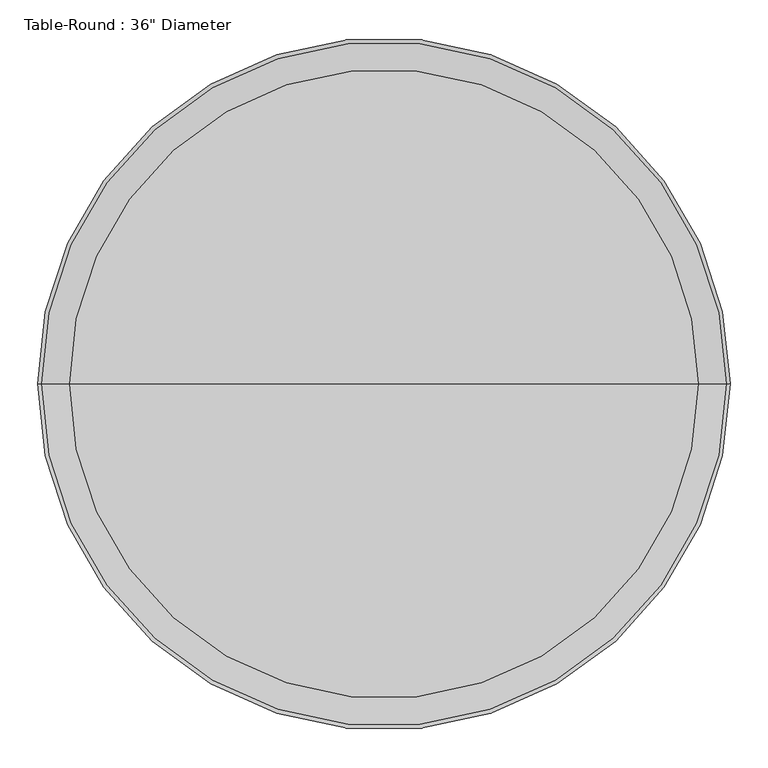
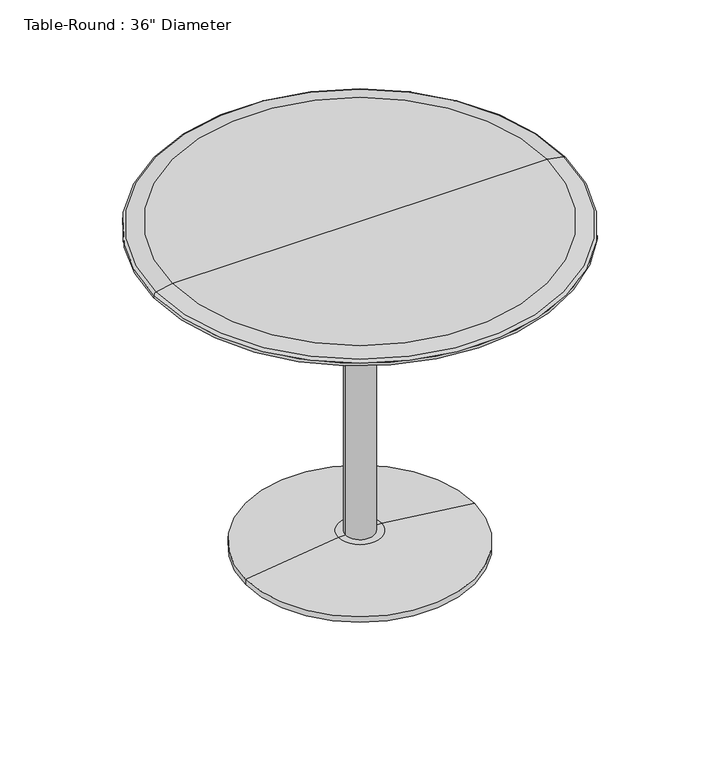
"""IFC4 building model written with IfcOpenShell, lengths in millimetres: furniture geometry."""

from ifc_helpers import new_model, si_unit, point, frame, origin, origin_2d, place, context, project, spatial, polyline, circle_curve, ellipse_curve, trimmed, segment, composite_curve, outline, extrude, source, transform, mapped, element, save
from ifc_brep_helpers import plane_surface, cylinder_surface, revolved_surface, advanced_brep


def furniture_c80d6d9c(model_context):
    return source(origin(), model_context, "Body", "SolidModel", [
        extrude(outline(composite_curve([segment(trimmed(circle_curve(origin_2d(), 31.75), [point((-31.75, 0.0))], [point((31.75, 0.0))], False, "CARTESIAN"), True, "CONTINUOUS"), segment(trimmed(circle_curve(origin_2d(), 31.75), [point((31.75, 0.0))], [point((-31.75, 0.0))], False, "CARTESIAN"), True, "CONTINUOUS")], self_intersect=False)), frame((0.0, 0.0, 38.1), z_axis=(0.0, 0.0, 1.0), x_axis=(1.0, 0.0, 0.0)), (0.0, 0.0, 1.0), 704.85),
        advanced_brep(
        [(0.0, 0.0, 742.95), (-457.2, 0.0, 742.95), (457.2, 0.0, 742.95), (415.3011364, 0.0, 762.0), (-415.3011364, 0.0, 762.0), (0.0, 0.0, 762.0), (451.9526659, 0.0, 755.5373465), (-451.9526659, 0.0, 755.5373465), (457.2, 0.0, 749.2838172), (-457.2, 0.0, 749.2838172)],
        [
            (0, 1),
            (1, 2, circle_curve(frame((0.0, 0.0, 742.95), z_axis=(0.0, 0.0, -1.0), x_axis=(-1.0, 0.0, 0.0)), 457.2)),
            (2, 0),
            (2, 1, circle_curve(frame((0.0, 0.0, 742.95), z_axis=(0.0, 0.0, -1.0), x_axis=(-1.0, 0.0, 0.0)), 457.2)),
            (3, 4, circle_curve(frame((0.0, 0.0, 762.0), z_axis=(0.0, 0.0, 1.0), x_axis=(-1.0, 0.0, 0.0)), 415.3011364)),
            (4, 5),
            (5, 3),
            (4, 3, circle_curve(frame((0.0, 0.0, 762.0), z_axis=(0.0, 0.0, 1.0), x_axis=(-1.0, 0.0, 0.0)), 415.3011364)),
            (6, 7, circle_curve(frame((0.0, 0.0, 755.5373465), z_axis=(0.0, 0.0, 1.0), x_axis=(-1.0, 0.0, 0.0)), 451.9526659)),
            (7, 4),
            (3, 6),
            (7, 6, circle_curve(frame((0.0, 0.0, 755.5373465), z_axis=(0.0, 0.0, 1.0), x_axis=(-1.0, 0.0, 0.0)), 451.9526659)),
            (8, 9, circle_curve(frame((0.0, 0.0, 749.2838172), z_axis=(0.0, 0.0, 1.0), x_axis=(-1.0, 0.0, 0.0)), 457.2)),
            (9, 7, circle_curve(frame((-450.85, 0.0, 749.2838172), z_axis=(0.0, 1.0, 0.0), x_axis=(1.0, 0.0, 0.0)), 6.35)),
            (6, 8, circle_curve(frame((450.85, 0.0, 749.2838172), z_axis=(0.0, 1.0, 0.0), x_axis=(-1.0, 0.0, 0.0)), 6.35)),
            (9, 8, circle_curve(frame((0.0, 0.0, 749.2838172), z_axis=(0.0, 0.0, 1.0), x_axis=(-1.0, 0.0, 0.0)), 457.2)),
            (1, 9),
            (8, 2),
        ],
        [
            plane_surface(frame((0.0, 0.0, 742.95), z_axis=(0.0, 0.0, -1.0), x_axis=(-1.0, 0.0, 0.0))),
            plane_surface(frame((0.0, 0.0, 762.0), z_axis=(0.0, 0.0, 1.0), x_axis=(-1.0, 0.0, 0.0))),
            revolved_surface(polyline([(-415.3011364, 0.0, 762.0), (-451.9526659, 0.0, 755.5373465)]), (0.0, 0.0, 838.2), (0.0, 0.0, -1.0)),
            revolved_surface(trimmed(ellipse_curve(frame((-450.85, 0.0, 749.2838172), z_axis=(0.0, -1.0, 0.0), x_axis=(1.0, 0.0, 0.0)), 6.35, 6.35), [point((-451.9526659, 0.0, 755.5373465))], [point((-457.2, 0.0, 749.2838172))], True, "CARTESIAN"), (0.0, 0.0, 838.2), (0.0, 0.0, -1.0)),
            cylinder_surface(frame((0.0, 0.0, 838.2), z_axis=(0.0, 0.0, -1.0), x_axis=(-1.0, 0.0, 0.0)), 457.2),
        ],
        [
            (0, [[1, 2, 3]]),
            (0, [[-3, 4, -1]]),
            (1, [[5, 6, 7]]),
            (1, [[8, -7, -6]]),
            (2, [[9, 10, -5, 11]]),
            (2, [[12, -11, -8, -10]]),
            (3, [[13, 14, -9, 15]]),
            (3, [[16, -15, -12, -14]]),
            (4, [[-2, 17, -13, 18]]),
            (4, [[-4, -18, -16, -17]]),
        ],
    ),
        advanced_brep(
        [(0.0, 0.0, 0.0), (-254.0, 0.0, 0.0), (254.0, 0.0, 0.0), (47.625, 0.0, 38.1), (-47.625, 0.0, 38.1), (0.0, 0.0, 38.1), (254.0, 0.0, 12.7), (-254.0, 0.0, 12.7)],
        [
            (0, 1),
            (1, 2, circle_curve(frame((0.0, 0.0, 0.0), z_axis=(0.0, 0.0, -1.0), x_axis=(-1.0, 0.0, 0.0)), 254.0)),
            (2, 0),
            (2, 1, circle_curve(frame((0.0, 0.0, 0.0), z_axis=(0.0, 0.0, -1.0), x_axis=(-1.0, 0.0, 0.0)), 254.0)),
            (3, 4, circle_curve(frame((0.0, 0.0, 38.1), z_axis=(0.0, 0.0, 1.0), x_axis=(-1.0, 0.0, 0.0)), 47.625)),
            (4, 5),
            (5, 3),
            (4, 3, circle_curve(frame((0.0, 0.0, 38.1), z_axis=(0.0, 0.0, 1.0), x_axis=(-1.0, 0.0, 0.0)), 47.625)),
            (6, 7, circle_curve(frame((0.0, 0.0, 12.7), z_axis=(0.0, 0.0, 1.0), x_axis=(-1.0, 0.0, 0.0)), 254.0)),
            (7, 4),
            (3, 6),
            (7, 6, circle_curve(frame((0.0, 0.0, 12.7), z_axis=(0.0, 0.0, 1.0), x_axis=(-1.0, 0.0, 0.0)), 254.0)),
            (1, 7),
            (6, 2),
        ],
        [
            plane_surface(frame((0.0, 0.0, 0.0), z_axis=(0.0, 0.0, -1.0), x_axis=(-1.0, 0.0, 0.0))),
            plane_surface(frame((0.0, 0.0, 38.1), z_axis=(0.0, 0.0, 1.0), x_axis=(-1.0, 0.0, 0.0))),
            revolved_surface(polyline([(-47.625, 0.0, 38.1), (-254.0, 0.0, 12.7)]), (0.0, 0.0, 215.9), (0.0, 0.0, -1.0)),
            cylinder_surface(frame((0.0, 0.0, 215.9), z_axis=(0.0, 0.0, -1.0), x_axis=(-1.0, 0.0, 0.0)), 254.0),
        ],
        [
            (0, [[1, 2, 3]]),
            (0, [[-3, 4, -1]]),
            (1, [[5, 6, 7]]),
            (1, [[8, -7, -6]]),
            (2, [[9, 10, -5, 11]]),
            (2, [[12, -11, -8, -10]]),
            (3, [[-2, 13, -9, 14]]),
            (3, [[-4, -14, -12, -13]]),
        ],
    ),
    ])


if __name__ == "__main__":
    model = new_model("IFC4")
    model_context = context("Model", 3, world=origin())
    ifc_project = project(units=[si_unit("LENGTHUNIT", "METRE", prefix="MILLI")], contexts=[model_context])
    site = spatial("IfcSite", under=ifc_project)
    building = spatial("IfcBuilding", under=site)
    placement = place(None, origin())
    furniture_shape = furniture_c80d6d9c(model_context)
    element("IfcFurniture", 1, ObjectType="Table-Round : 36\" Diameter", at=placement, inside=building, context=model_context, shape_type="MappedRepresentation", body=[
        mapped(furniture_shape, transform((0.0, 0.0, 0.0), x_axis=(1.0, 0.0, 0.0), y_axis=(0.0, 1.0, 0.0), z_axis=(0.0, 0.0, 1.0))),
    ])
    save(model, "model.ifc")

# Revit data of these elements
# Type "Table-Round : 36\" Diameter"
#   Assembly Code = "E2020200"
#   Base Radius = 0' - 10"
#   Height = 2' - 6"
#   Radius = 1' - 6"
#   Base Material = Steel, Chrome Plated
#   Top Material = Birch
#   Default Elevation = 0
# Element 1 (IfcFurniture, "Table-Round : 36\" Diameter")
#   Materials on its faces: "Steel, Chrome Plated", "Birch"
# Materials
#   "Steel, Chrome Plated": class "Metal", colour RGB 17 17 17, transparency 0, Description = "Chromiuim plated steel", Cost = 0
#   "Birch": class "Wood", colour RGB 210 159 95, transparency 0, Description = "Betula Alleghaniensis", Cost = 0
